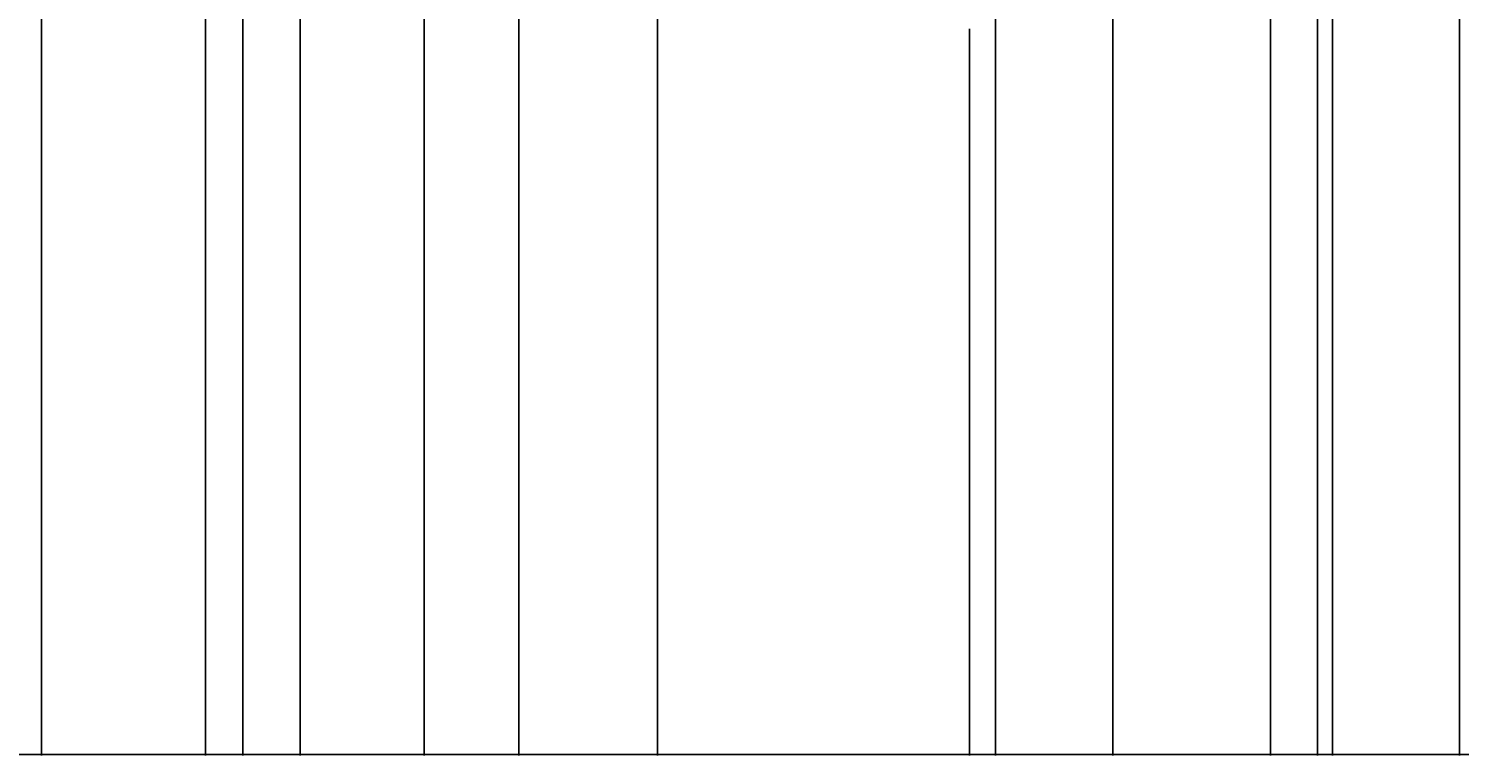
# Model space of a CAD drawing. Units: inches. Extents: x -742 to 1386, y -64 to 951.
# Tile 3 of 8: x 43 to 376, y -64 to 106. Entities that reach past the tile are written whole.
import ezdxf

# ---------------------------------------------------------------- set-up
doc = ezdxf.new("R2010")
doc.units = ezdxf.units.IN
doc.header["$MEASUREMENT"] = 0
doc.layers.add('A-ANNO-DIMS', color=2, linetype='Continuous', lineweight=18)
doc.styles.get("Standard").update_dxf_attribs({"font": 'arial.ttf'})
doc.dimstyles.get("Standard").update_dxf_attribs({"dimtxt": 0.18, "dimasz": 0.18, "dimexe": 0.18, "dimexo": 0.0625, "dimgap": 0.09, "dimtad": 0, "dimtih": 1, "dimtoh": 1, "dimdec": 4, "dimzin": 0, "dimdsep": 46, "dimtxsty": 'Standard', "dimcen": 0.09, "dimadec": 0, "dimazin": 0, "dimtfac": 1, "dimtdec": 4, "dimtofl": 0, "dimtmove": 0, "dimatfit": 3, "dimfxl": 1, "dimtolj": 1, "dimtzin": 0, "dimarcsym": 0})

# ---------------------------------------------------------------- blocks, each defined once
blk = doc.blocks.new('*D14')
at = {"layer": 'A-ANNO-DIMS', "color": 0, "lineweight": -2, "transparency": 16777216}
for p, q in [((-37.77, 105.68), (-37.77, -63.58)), ((262.23, 105.68), (262.23, -63.58)), ((-37.59, -63.4), (111.94, -63.4)), ((262.05, -63.4), (112.52, -63.4))]:
    blk.add_line(p, q, dxfattribs=at)
at = {"layer": 'A-ANNO-DIMS', "color": 0, "transparency": 16777216}
for points in [[(-37.59, -63.37), (-37.59, -63.43), (-37.77, -63.4)], [(262.05, -63.37), (262.05, -63.43), (262.23, -63.4)]]:
    blk.add_solid(points, dxfattribs=at)
at = {"layer": 'Defpoints', "color": 0, "transparency": 16777216}
for p in [(-37.77, 105.74), (262.23, 105.74), (262.23, -63.4)]:
    blk.add_point(p, dxfattribs=at)
at = {"layer": 'A-ANNO-DIMS', "color": 0, "transparency": 16777216, "insert": (112.23, -63.4), "char_height": 0.18, "attachment_point": 5}
blk.add_mtext('\\A1;300', dxfattribs=at)
blk = doc.blocks.new('*D15')
at = {"layer": 'A-ANNO-DIMS', "color": 0, "lineweight": -2, "transparency": 16777216}
for p, q in [((262.23, 105.68), (262.23, -63.58)), ((382.23, 105.68), (382.23, -63.58)), ((262.41, -63.4), (321.95, -63.4)), ((382.05, -63.4), (322.51, -63.4))]:
    blk.add_line(p, q, dxfattribs=at)
at = {"layer": 'A-ANNO-DIMS', "color": 0, "transparency": 16777216}
for points in [[(262.41, -63.37), (262.41, -63.43), (262.23, -63.4)], [(382.05, -63.37), (382.05, -63.43), (382.23, -63.4)]]:
    blk.add_solid(points, dxfattribs=at)
at = {"layer": 'Defpoints', "color": 0, "transparency": 16777216}
for p in [(262.23, 105.74), (382.23, 105.74), (382.23, -63.4)]:
    blk.add_point(p, dxfattribs=at)
at = {"layer": 'A-ANNO-DIMS', "color": 0, "transparency": 16777216, "insert": (322.23, -63.4), "char_height": 0.18, "attachment_point": 5}
blk.add_mtext('\\A1;120', dxfattribs=at)
blk = doc.blocks.new('*D20')
at = {"layer": 'A-ANNO-DIMS', "color": 0, "lineweight": -2, "transparency": 16777216}
for p, q in [((40.23, 141.68), (40.23, -63.58)), ((46.23, 141.68), (46.23, -63.58)), ((40.41, -63.4), (43.08, -63.4)), ((46.05, -63.4), (43.38, -63.4))]:
    blk.add_line(p, q, dxfattribs=at)
at = {"layer": 'A-ANNO-DIMS', "color": 0, "transparency": 16777216}
for points in [[(40.41, -63.37), (40.41, -63.43), (40.23, -63.4)], [(46.05, -63.37), (46.05, -63.43), (46.23, -63.4)]]:
    blk.add_solid(points, dxfattribs=at)
at = {"layer": 'Defpoints', "color": 0, "transparency": 16777216}
for p in [(40.23, 141.74), (46.23, 141.74), (46.23, -63.4)]:
    blk.add_point(p, dxfattribs=at)
at = {"layer": 'A-ANNO-DIMS', "color": 0, "transparency": 16777216, "insert": (43.23, -63.4), "char_height": 0.18, "attachment_point": 5}
blk.add_mtext('\\A1;6', dxfattribs=at)
blk = doc.blocks.new('*D25')
at = {"layer": 'A-ANNO-DIMS', "color": 0, "lineweight": -2, "transparency": 16777216}
for p, q in [((46.23, 178.68), (46.23, -63.58)), ((93.11, 178.68), (93.11, -63.58)), ((46.41, -63.4), (69.27, -63.4)), ((92.93, -63.4), (70.07, -63.4))]:
    blk.add_line(p, q, dxfattribs=at)
at = {"layer": 'A-ANNO-DIMS', "color": 0, "transparency": 16777216}
for points in [[(46.41, -63.37), (46.41, -63.43), (46.23, -63.4)], [(92.93, -63.37), (92.93, -63.43), (93.11, -63.4)]]:
    blk.add_solid(points, dxfattribs=at)
at = {"layer": 'Defpoints', "color": 0, "transparency": 16777216}
for p in [(46.23, 178.74), (93.11, 178.74), (93.11, -63.4)]:
    blk.add_point(p, dxfattribs=at)
at = {"layer": 'A-ANNO-DIMS', "color": 0, "transparency": 16777216, "insert": (69.67, -63.4), "char_height": 0.18, "attachment_point": 5}
blk.add_mtext('\\A1;46.88', dxfattribs=at)
blk = doc.blocks.new('*D26')
at = {"layer": 'A-ANNO-DIMS', "color": 0, "lineweight": -2, "transparency": 16777216}
for p, q in [((84.43, 232.16), (84.43, -63.58)), ((46.23, 225.68), (46.23, -63.58)), ((46.41, -63.4), (65, -63.4)), ((84.25, -63.4), (65.65, -63.4))]:
    blk.add_line(p, q, dxfattribs=at)
at = {"layer": 'A-ANNO-DIMS', "color": 0, "transparency": 16777216}
for points in [[(46.41, -63.37), (46.41, -63.43), (46.23, -63.4)], [(84.25, -63.37), (84.25, -63.43), (84.43, -63.4)]]:
    blk.add_solid(points, dxfattribs=at)
at = {"layer": 'Defpoints', "color": 0, "transparency": 16777216}
for p in [(84.43, 232.23), (46.23, 225.74), (84.43, -63.4)]:
    blk.add_point(p, dxfattribs=at)
at = {"layer": 'A-ANNO-DIMS', "color": 0, "transparency": 16777216, "insert": (65.33, -63.4), "char_height": 0.18, "attachment_point": 5}
blk.add_mtext('\\A1;38.2', dxfattribs=at)
blk = doc.blocks.new('*D27')
at = {"layer": 'A-ANNO-DIMS', "color": 0, "lineweight": -2, "transparency": 16777216}
for p, q in [((106.41, 232.16), (106.41, -63.58)), ((135.32, 232.16), (135.32, -63.58)), ((106.59, -63.4), (120.49, -63.4)), ((135.14, -63.4), (121.25, -63.4))]:
    blk.add_line(p, q, dxfattribs=at)
at = {"layer": 'A-ANNO-DIMS', "color": 0, "transparency": 16777216}
for points in [[(106.59, -63.37), (106.59, -63.43), (106.41, -63.4)], [(135.14, -63.37), (135.14, -63.43), (135.32, -63.4)]]:
    blk.add_solid(points, dxfattribs=at)
at = {"layer": 'Defpoints', "color": 0, "transparency": 16777216}
for p in [(106.41, 232.23), (135.32, 232.23), (135.32, -63.4)]:
    blk.add_point(p, dxfattribs=at)
at = {"layer": 'A-ANNO-DIMS', "color": 0, "transparency": 16777216, "insert": (120.87, -63.4), "char_height": 0.18, "attachment_point": 5}
blk.add_mtext('\\A1;28.91', dxfattribs=at)
blk = doc.blocks.new('*D28')
at = {"layer": 'A-ANNO-DIMS', "color": 0, "lineweight": -2, "transparency": 16777216}
for p, q in [((157.31, 232.16), (157.31, -63.58)), ((189.57, 232.16), (189.57, -63.58)), ((157.49, -63.4), (172.98, -63.4)), ((189.39, -63.4), (173.91, -63.4))]:
    blk.add_line(p, q, dxfattribs=at)
at = {"layer": 'A-ANNO-DIMS', "color": 0, "transparency": 16777216}
for points in [[(157.49, -63.37), (157.49, -63.43), (157.31, -63.4)], [(189.39, -63.37), (189.39, -63.43), (189.57, -63.4)]]:
    blk.add_solid(points, dxfattribs=at)
at = {"layer": 'Defpoints', "color": 0, "transparency": 16777216}
for p in [(157.31, 232.23), (189.57, 232.23), (189.57, -63.4)]:
    blk.add_point(p, dxfattribs=at)
at = {"layer": 'A-ANNO-DIMS', "color": 0, "transparency": 16777216, "insert": (173.44, -63.4), "char_height": 0.18, "attachment_point": 5}
blk.add_mtext('\\A1;32.263', dxfattribs=at)
blk = doc.blocks.new('*D33')
at = {"layer": 'A-ANNO-DIMS', "color": 0, "lineweight": -2, "transparency": 16777216}
for p, q in [((268.23, 199.77), (268.23, -63.58)), ((332.25, 199.77), (332.25, -63.58)), ((268.41, -63.4), (299.84, -63.4)), ((332.07, -63.4), (300.63, -63.4))]:
    blk.add_line(p, q, dxfattribs=at)
at = {"layer": 'A-ANNO-DIMS', "color": 0, "transparency": 16777216}
for points in [[(268.41, -63.37), (268.41, -63.43), (268.23, -63.4)], [(332.07, -63.37), (332.07, -63.43), (332.25, -63.4)]]:
    blk.add_solid(points, dxfattribs=at)
at = {"layer": 'Defpoints', "color": 0, "transparency": 16777216}
for p in [(268.23, 199.83), (332.25, 199.83), (332.25, -63.4)]:
    blk.add_point(p, dxfattribs=at)
at = {"layer": 'A-ANNO-DIMS', "color": 0, "transparency": 16777216, "insert": (300.24, -63.4), "char_height": 0.18, "attachment_point": 5}
blk.add_mtext('\\A1;64.02', dxfattribs=at)
blk = doc.blocks.new('*D34')
at = {"layer": 'A-ANNO-DIMS', "color": 0, "lineweight": -2, "transparency": 16777216}
for p, q in [((332.25, 199.77), (332.25, -63.58)), ((343.24, 199.77), (343.24, -63.58)), ((332.43, -63.4), (337.29, -63.4)), ((343.06, -63.4), (338.2, -63.4))]:
    blk.add_line(p, q, dxfattribs=at)
at = {"layer": 'A-ANNO-DIMS', "color": 0, "transparency": 16777216}
for points in [[(332.43, -63.37), (332.43, -63.43), (332.25, -63.4)], [(343.06, -63.37), (343.06, -63.43), (343.24, -63.4)]]:
    blk.add_solid(points, dxfattribs=at)
at = {"layer": 'Defpoints', "color": 0, "transparency": 16777216}
for p in [(332.25, 199.83), (343.24, 199.83), (343.24, -63.4)]:
    blk.add_point(p, dxfattribs=at)
at = {"layer": 'A-ANNO-DIMS', "color": 0, "transparency": 16777216, "insert": (337.75, -63.4), "char_height": 0.18, "attachment_point": 5}
blk.add_mtext('\\A1;10.995', dxfattribs=at)
blk = doc.blocks.new('*D35')
at = {"layer": 'A-ANNO-DIMS', "color": 0, "lineweight": -2, "transparency": 16777216}
for p, q in [((343.24, 199.77), (343.24, -63.58)), ((376.23, 199.77), (376.23, -63.58)), ((343.42, -63.4), (359.27, -63.4)), ((376.05, -63.4), (360.2, -63.4))]:
    blk.add_line(p, q, dxfattribs=at)
at = {"layer": 'A-ANNO-DIMS', "color": 0, "transparency": 16777216}
for points in [[(343.42, -63.37), (343.42, -63.43), (343.24, -63.4)], [(376.05, -63.37), (376.05, -63.43), (376.23, -63.4)]]:
    blk.add_solid(points, dxfattribs=at)
at = {"layer": 'Defpoints', "color": 0, "transparency": 16777216}
for p in [(343.24, 199.83), (376.23, 199.83), (376.23, -63.4)]:
    blk.add_point(p, dxfattribs=at)
at = {"layer": 'A-ANNO-DIMS', "color": 0, "transparency": 16777216, "insert": (359.74, -63.4), "char_height": 0.18, "attachment_point": 5}
blk.add_mtext('\\A1;32.985', dxfattribs=at)
blk = doc.blocks.new('*D37')
at = {"layer": 'A-ANNO-DIMS', "color": 0, "lineweight": -2, "transparency": 16777216}
for p, q in [((268.23, 326.79), (268.23, -63.58)), ((295.56, 326.79), (295.56, -63.58)), ((268.41, -63.4), (281.43, -63.4)), ((295.38, -63.4), (282.36, -63.4))]:
    blk.add_line(p, q, dxfattribs=at)
at = {"layer": 'A-ANNO-DIMS', "color": 0, "transparency": 16777216}
for points in [[(268.41, -63.37), (268.41, -63.43), (268.23, -63.4)], [(295.38, -63.37), (295.38, -63.43), (295.56, -63.4)]]:
    blk.add_solid(points, dxfattribs=at)
at = {"layer": 'Defpoints', "color": 0, "transparency": 16777216}
for p in [(268.23, 326.85), (295.56, 326.85), (295.56, -63.4)]:
    blk.add_point(p, dxfattribs=at)
at = {"layer": 'A-ANNO-DIMS', "color": 0, "transparency": 16777216, "insert": (281.9, -63.4), "char_height": 0.18, "attachment_point": 5}
blk.add_mtext('\\A1;27.337', dxfattribs=at)
blk = doc.blocks.new('*D38')
at = {"layer": 'A-ANNO-DIMS', "color": 0, "lineweight": -2, "transparency": 16777216}
for p, q in [((295.56, 326.79), (295.56, -63.58)), ((346.7, 326.79), (346.7, -63.58)), ((295.74, -63.4), (320.74, -63.4)), ((346.52, -63.4), (321.52, -63.4))]:
    blk.add_line(p, q, dxfattribs=at)
at = {"layer": 'A-ANNO-DIMS', "color": 0, "transparency": 16777216}
for points in [[(295.74, -63.37), (295.74, -63.43), (295.56, -63.4)], [(346.52, -63.37), (346.52, -63.43), (346.7, -63.4)]]:
    blk.add_solid(points, dxfattribs=at)
at = {"layer": 'Defpoints', "color": 0, "transparency": 16777216}
for p in [(295.56, 326.85), (346.7, 326.85), (346.7, -63.4)]:
    blk.add_point(p, dxfattribs=at)
at = {"layer": 'A-ANNO-DIMS', "color": 0, "transparency": 16777216, "insert": (321.13, -63.4), "char_height": 0.18, "attachment_point": 5}
blk.add_mtext('\\A1;51.13', dxfattribs=at)

msp = doc.modelspace()

# ---------------------------------------------------------------- dimensions: what is measured, and where the dimension line sits
at = {"layer": 'A-ANNO-DIMS'}
for base, p1, p2, override, picture, middle in [((295.5643, -63.3971), (268.2276, 326.8548), (295.5643, 326.8548), {"dimdec": 3, "dimlfac": 1, "dimrnd": 0, "dimzin": 0, "dimdsep": 46, "dimlunit": 2}, '*D37', (281.896, -63.3971)), ((346.6973, -63.3971), (295.5643, 326.8548), (346.6973, 326.8548), {"dimdec": 2, "dimlfac": 1, "dimrnd": 0, "dimzin": 0, "dimdsep": 46, "dimlunit": 2}, '*D38', (321.1308, -63.3971)), ((84.4263, -63.3971), (46.2276, 225.7399), (84.4263, 232.2254), {"dimdec": 1, "dimlfac": 1, "dimrnd": 0, "dimzin": 0, "dimdsep": 46, "dimlunit": 2}, '*D26', (65.3269, -63.3971)), ((135.3236, -63.3971), (106.4136, 232.2254), (135.3236, 232.2254), {"dimdec": 2, "dimlfac": 1, "dimrnd": 0, "dimzin": 0, "dimdsep": 46, "dimlunit": 2}, '*D27', (120.8686, -63.3971)), ((189.5743, -63.3971), (157.3109, 232.2254), (189.5743, 232.2254), {"dimdec": 3, "dimlfac": 1, "dimrnd": 0, "dimzin": 0, "dimdsep": 46, "dimlunit": 2}, '*D28', (173.4426, -63.3971)), ((332.2479, -63.3971), (268.2276, 199.8339), (332.2479, 199.8339), {"dimdec": 2, "dimlfac": 1, "dimrnd": 0, "dimzin": 0, "dimdsep": 46, "dimlunit": 2}, '*D33', (300.2378, -63.3971)), ((343.2429, -63.3971), (332.2479, 199.8339), (343.2429, 199.8339), {"dimdec": 3, "dimlfac": 1, "dimrnd": 0, "dimzin": 0, "dimdsep": 46, "dimlunit": 2}, '*D34', (337.7454, -63.3971)), ((376.2276, -63.3971), (343.2429, 199.8339), (376.2276, 199.8339), {"dimdec": 3, "dimlfac": 1, "dimrnd": 0, "dimzin": 0, "dimdsep": 46, "dimlunit": 2}, '*D35', (359.7352, -63.3971)), ((93.1117, -63.3971), (46.2276, 178.7399), (93.1117, 178.7399), {"dimdec": 2, "dimlfac": 1, "dimrnd": 0, "dimzin": 0, "dimdsep": 46, "dimlunit": 2}, '*D25', (69.6697, -63.3971)), ((46.2276, -63.3971), (40.2276, 141.7399), (46.2276, 141.7399), {"dimdec": 0, "dimlfac": 1, "dimrnd": 0, "dimzin": 0, "dimdsep": 46, "dimlunit": 2}, '*D20', (43.2276, -63.3971)), ((262.2276, -63.3971), (-37.7724, 105.7399), (262.2276, 105.7399), {"dimdec": 0, "dimlfac": 1, "dimrnd": 0, "dimzin": 0, "dimdsep": 46, "dimlunit": 2}, '*D14', (112.2276, -63.3971)), ((382.2276, -63.3971), (262.2276, 105.7399), (382.2276, 105.7399), {"dimdec": 0, "dimlfac": 1, "dimrnd": 0, "dimzin": 0, "dimdsep": 46, "dimlunit": 2}, '*D15', (322.2276, -63.3971))]:
    dim = msp.add_linear_dim(base=base, p1=p1, p2=p2, dimstyle='Standard', override=override, dxfattribs=at)
    dim.commit()
    dim.dimension.update_dxf_attribs({"geometry": picture, "text_midpoint": middle})

doc.saveas('drawing.dxf')
